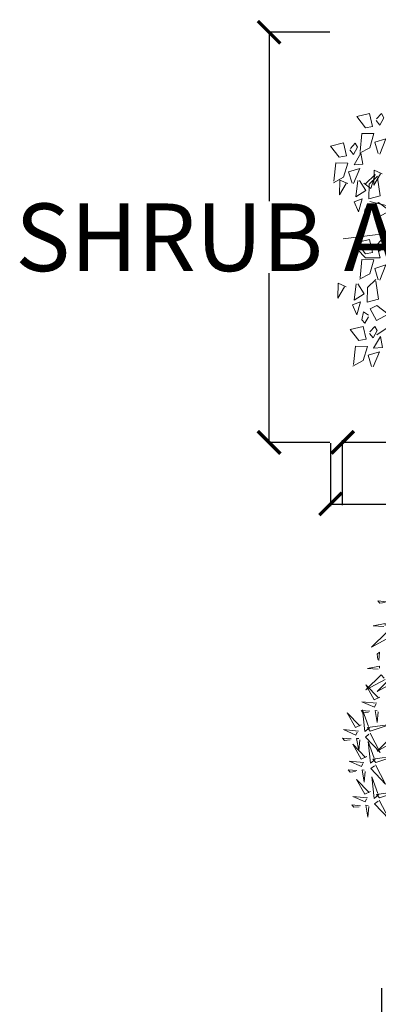
# Model space of a CAD drawing. Units: inches. Extents: x 1704 to 6393, y -157 to 1172.
# Tile 2 of 122: x 1866 to 1898, y -5 to 82. Entities that reach past the tile are written whole.
import ezdxf

# ---------------------------------------------------------------- set-up
doc = ezdxf.new("R2010")
doc.units = ezdxf.units.IN
doc.header["$MEASUREMENT"] = 0
for name, color, linetype, lineweight in [('A-ANNO-DIMS', 7, 'Continuous', 13), ('L-shrub', 74, 'Continuous', 18), ('L-tree', 102, 'Continuous', 18)]:
    doc.layers.add(name, color=color, linetype=linetype, lineweight=lineweight)
doc.styles.get("Standard").update_dxf_attribs({"font": 'arial.ttf'})
doc.dimstyles.get("Standard").update_dxf_attribs({"dimtxt": 6, "dimasz": 2, "dimexe": 0.18, "dimexo": 0.0625, "dimgap": 0.09, "dimtad": 0, "dimtih": 1, "dimtoh": 1, "dimdec": 1, "dimzin": 0, "dimdsep": 46, "dimlunit": 3, "dimtxsty": 'Standard', "dimblk": 'ARCHTICK', "dimcen": 0.09, "dimadec": 0, "dimazin": 0, "dimtfac": 1, "dimtdec": 1, "dimtofl": 0, "dimtmove": 0, "dimatfit": 3, "dimfxl": 1, "dimtolj": 1, "dimtzin": 0, "dimarcsym": 0})

# ---------------------------------------------------------------- blocks, each defined once
blk = doc.blocks.new('bamboo')
at = {"layer": 'L-shrub'}
for points in [[(-549.8, -1084.4), (-473.4, -1224.8), (-583.8, -1113.5), (-558.3, -1091.7)], [(-222.2, -1043.5), (-145.8, -1183.9), (-256.1, -1072.6), (-230.7, -1050.8)], [(214.7, -1043.5), (291.1, -1183.9), (180.8, -1072.6), (206.2, -1050.8)], [(376.8, -1193.4), (327.4, -1045.8), (350.9, -1214.7), (376.8, -1193.4)], [(636.2, -1166.1), (586.8, -1018.5), (610.3, -1187.4), (636.2, -1166.1)], [(-807.6, -1115.7), (-813.6, -1178.6), (-796.4, -1164.4), (-800.5, -1124.4)], [(-624.9, -1134.2), (-630.9, -1213), (-648, -1124.6), (-632.2, -1125.7)], [(-235.8, -1125.3), (-159.4, -1265.7), (-269.7, -1154.4), (-244.3, -1132.6)], [(144.7, -1234.3), (95.3, -1086.7), (118.8, -1255.6), (144.7, -1234.3)], [(392.5, -1194.9), (534.4, -1121.4), (420.9, -1229.4), (399.6, -1203.5)], [(651.9, -1167.6), (793.8, -1094.1), (680.3, -1202.1), (659, -1176.3)], [(-373.9, -1170.4), (-436.9, -1165.7), (-422.4, -1182.6), (-382.4, -1177.7)], [(-310.9, -1175.1), (-316.9, -1253.9), (-334, -1165.5), (-318.2, -1166.6)], [(-106.2, -1164.9), (-86.3, -1206.5), (-195.3, -1267.4), (-99.1, -1173.5)], [(-60.5, -1185.2), (-71, -1295.3), (-30.6, -1204), (-53.4, -1193.8)], [(3.9, -1175.6), (82.5, -1183.2), (-6.2, -1198.4), (-4.7, -1182.7)], [(160.4, -1235.8), (302.3, -1162.3), (188.8, -1270.3), (167.5, -1244.4)], [(352.4, -1199), (380.9, -1233.5), (220.7, -1249.7), (343.8, -1206.1)], [(611.8, -1171.7), (640.3, -1206.2), (480.1, -1222.4), (603.2, -1178.8)], [(120.3, -1239.9), (148.8, -1274.4), (-11.4, -1290.6), (111.7, -1247)], [(-2.1, -1238.5), (-8.1, -1301.4), (9.1, -1287.1), (5, -1247.1)], [(98.6, -1301.3), (118.4, -1342.9), (9.5, -1403.7), (105.7, -1309.9)], [(330.7, -1260.4), (350.5, -1301.9), (241.6, -1362.8), (337.8, -1269)], [(376.4, -1280.6), (365.9, -1390.7), (406.3, -1299.4), (383.5, -1289.3)], [(440.8, -1271), (519.4, -1278.6), (430.7, -1293.8), (432.2, -1278.1)], [(590.1, -1233.1), (609.9, -1274.7), (501, -1335.5), (597.2, -1241.7)], [(635.8, -1253.4), (625.3, -1363.4), (665.7, -1272.1), (642.9, -1262)], [(700.2, -1243.7), (778.8, -1251.3), (690.1, -1266.6), (691.6, -1250.8)], [(144.3, -1321.5), (133.8, -1431.6), (174.2, -1340.3), (151.4, -1330.2)], [(202.7, -1374.8), (196.7, -1437.7), (213.9, -1423.5), (209.8, -1383.4)], [(208.7, -1311.9), (287.3, -1319.5), (198.6, -1334.7), (200.1, -1319)], [(434.8, -1333.9), (428.8, -1396.8), (446, -1382.6), (441.9, -1342.5)], [(694.2, -1306.6), (688.2, -1369.5), (705.4, -1355.3), (701.3, -1315.3)]]:
    blk.add_lwpolyline(points, dxfattribs=at)
blk = doc.blocks.new('flower shrub 3')
at = {"layer": 'L-shrub'}
for p, q in [((10.1, -195.8), (26, -191.4)), ((14.6, -220.7), (10.1, -195.8)), ((26, -191.4), (25.9, -211.7)), ((25.9, -211.7), (14.5, -223))]:
    blk.add_line(p, q, dxfattribs=at)
for points in [[(-2.5, -5.1), (-51.6, -205.9)], [(7.3, -10), (132.3, -196.1)], [(-12.3, -147.2), (-0.1, -242.7)], [(-163.4, -197.2), (-157.2, -192), (-167.4, -186.6), (-173, -189.7), (-165.6, -196.5)], [(-117.8, -194.2), (-133.4, -199), (-138.2, -183.5), (-117.2, -192.1)], [(-89.9, -188.6), (-94.8, -199.8), (-74.4, -200.3), (-90, -190.9)], [(-50.4, -193.8), (-38.7, -178.3), (-30.1, -194.3), (-46.1, -202.9), (-50.4, -193.8)], [(10.5, -197.2), (16.8, -192), (6.6, -186.6), (1, -189.7), (8.3, -196.5)], [(56.1, -194.2), (40.6, -199), (35.8, -183.5), (56.8, -192.1)], [(91.9, -196.1), (103.6, -180.6), (112.3, -196.6), (96.2, -205.2), (91.9, -196.1)], [(150.8, -200.5), (149.6, -188.4), (134.7, -191.1), (150.8, -200.5)], [(-153.6, -211.9), (-169, -223.8), (-173.1, -206.1), (-155.4, -201.9), (-153.6, -211.9)], [(-120.5, -219.3), (-145.6, -216.6), (-145.5, -200.2), (-126, -205.9), (-118.3, -219.9)], [(-77, -213.9), (-69.5, -204.4), (-88.9, -198.6), (-76.3, -211.7)], [(-84.3, -195.1), (-59.4, -191.3), (-55.3, -207.2), (-75.6, -206.7), (-86.6, -195.1)], [(20.3, -211.9), (5, -223.8), (0.8, -206.1), (18.5, -201.9), (20.3, -211.9)], [(53.4, -219.3), (28.3, -216.6), (28.5, -200.2), (48, -205.9), (55.6, -219.9)], [(58, -197.4), (83, -193.6), (87.1, -209.5), (66.7, -208.9), (55.7, -197.3)], [(130.2, -206.2), (136.5, -201), (126.3, -195.6), (120.7, -198.7), (128.1, -205.6)], [(175.9, -203.3), (160.3, -208.1), (155.5, -192.5), (176.5, -201.1)], [(-102.2, -227.6), (-103.4, -215.5), (-118.3, -218.1), (-102.2, -227.6)], [(-80.5, -220.1), (-66.7, -211.4), (-58, -225.2), (-80.5, -222.3)], [(-55.5, -216.2), (-51.3, -227.6), (-37.6, -221.2), (-55.5, -216.2)], [(-37.1, -205.4), (-41.8, -212.1), (-30.6, -214.6), (-26, -210.3), (-34.9, -205.5)], [(61.8, -222.3), (75.6, -213.7), (84.3, -227.4), (61.8, -224.6)], [(105.2, -207.7), (100.5, -214.3), (111.7, -216.9), (116.3, -212.5), (107.4, -207.8)], [(140, -220.9), (124.7, -232.8), (120.5, -215.1), (138.3, -210.9), (140, -220.9)], [(173.2, -228.3), (148, -225.6), (148.2, -209.2), (167.7, -214.9), (175.3, -229)], [(-122.8, -233.3), (-116.5, -228.1), (-126.7, -222.7), (-132.3, -225.8), (-124.9, -232.6)], [(-77.1, -230.3), (-92.7, -235.1), (-97.5, -219.6), (-76.5, -228.2)], [(86.8, -218.5), (91, -229.9), (104.7, -223.5), (86.8, -218.5)], [(-113, -248), (-128.3, -259.9), (-132.5, -242.2), (-114.7, -238), (-113, -248)], [(-79.8, -255.4), (-105, -252.7), (-104.8, -236.3), (-85.3, -242), (-77.7, -256)], [(-76.4, -236), (-81.2, -247.1), (-60.9, -247.7), (-76.4, -238.2)], [(65.9, -238.2), (61.1, -249.4), (81.4, -249.9), (65.9, -240.5)]]:
    blk.add_lwpolyline(points, dxfattribs=at)
blk = doc.blocks.new('_ArchTick')
at = {"color": 0, "linetype": 'ByBlock', "const_width": 0.15}
blk.add_lwpolyline([(-0.5, -0.5), (0.5, 0.5)], dxfattribs=at)
blk = doc.blocks.new('*D71')
at = {"layer": 'A-ANNO-DIMS', "color": 0, "lineweight": -2, "transparency": 16777216}
for p, q in [((1894.896, 38.988), (1894.896, 44.734)), ((1894.896, 44.554), (1908.656, 44.554)), ((1931.183, 44.554), (1917.422, 44.554)), ((1931.183, 38.988), (1931.183, 44.734))]:
    blk.add_line(p, q, dxfattribs=at)
at = {"layer": 'Defpoints', "color": 0, "lineweight": -3, "transparency": 16777216}
for p in [(1931.183, 44.554), (1894.896, 38.926), (1931.183, 38.926)]:
    blk.add_point(p, dxfattribs=at)
at = {"layer": 'A-ANNO-DIMS', "color": 0, "lineweight": -2, "transparency": 16777216, "xscale": 2, "yscale": 2, "zscale": 2, "rotation": 180}
blk.add_blockref('_ArchTick', (1894.896, 44.554), dxfattribs=at)
at = {"layer": 'A-ANNO-DIMS', "color": 0, "lineweight": -2, "transparency": 16777216, "xscale": 2, "yscale": 2, "zscale": 2}
blk.add_blockref('_ArchTick', (1931.183, 44.554), dxfattribs=at)
at = {"layer": 'A-ANNO-DIMS', "color": 0, "transparency": 16777216, "insert": (1913.039, 44.554), "char_height": 6, "attachment_point": 5}
blk.add_mtext('\\A1;36', dxfattribs=at)
blk = doc.blocks.new('*D86')
at = {"layer": 'A-ANNO-DIMS', "color": 0, "lineweight": -2, "transparency": 16777216}
for p, q in [((1893.767, 80.936), (1888.19, 80.936)), ((1888.37, 80.936), (1888.37, 65.933)), ((1888.37, 44.542), (1888.37, 59.544)), ((1893.767, 44.542), (1888.19, 44.542))]:
    blk.add_line(p, q, dxfattribs=at)
at = {"layer": 'Defpoints', "color": 0, "lineweight": -3, "transparency": 16777216}
for p in [(1893.829, 80.936), (1888.37, 44.542), (1893.829, 44.542)]:
    blk.add_point(p, dxfattribs=at)
at = {"layer": 'A-ANNO-DIMS', "color": 0, "lineweight": -2, "transparency": 16777216, "xscale": 2, "yscale": 2, "zscale": 2}
for p, rotation in [((1888.37, 80.936), 90), ((1888.37, 44.542), 270)]:
    blk.add_blockref('_ArchTick', p, dxfattribs=dict(at, rotation=rotation))
at = {"layer": 'A-ANNO-DIMS', "color": 0, "transparency": 16777216, "insert": (1888.37, 62.739), "char_height": 6, "attachment_point": 5}
blk.add_mtext('\\A1;SHRUB A 36', dxfattribs=at)
blk = doc.blocks.new('*D87')
at = {"layer": 'A-ANNO-DIMS', "color": 0, "lineweight": -2, "transparency": 16777216}
for p, q in [((1893.829, 44.479), (1893.829, 38.903)), ((1928.523, 44.479), (1928.523, 38.903)), ((1893.829, 39.083), (1906.768, 39.083)), ((1928.523, 39.083), (1915.584, 39.083))]:
    blk.add_line(p, q, dxfattribs=at)
at = {"layer": 'Defpoints', "color": 0, "lineweight": -3, "transparency": 16777216}
for p in [(1893.829, 44.542), (1928.523, 44.542), (1928.523, 39.083)]:
    blk.add_point(p, dxfattribs=at)
at = {"layer": 'A-ANNO-DIMS', "color": 0, "lineweight": -2, "transparency": 16777216, "xscale": 2, "yscale": 2, "zscale": 2, "rotation": 180}
blk.add_blockref('_ArchTick', (1893.829, 39.083), dxfattribs=at)
at = {"layer": 'A-ANNO-DIMS', "color": 0, "lineweight": -2, "transparency": 16777216, "xscale": 2, "yscale": 2, "zscale": 2}
blk.add_blockref('_ArchTick', (1928.523, 39.083), dxfattribs=at)
at = {"layer": 'A-ANNO-DIMS', "color": 0, "transparency": 16777216, "insert": (1911.176, 39.083), "char_height": 6, "attachment_point": 5}
blk.add_mtext('\\A1;35', dxfattribs=at)
blk = doc.blocks.new('*D90')
at = {"layer": 'A-ANNO-DIMS', "color": 0, "lineweight": -2, "transparency": 16777216}
for p, q in [((1898.349, -3.85), (1898.349, -64.967)), ((2723.349, -3.85), (2723.349, -64.967)), ((1898.349, -64.787), (2304.104, -64.787)), ((2723.349, -64.787), (2317.593, -64.787))]:
    blk.add_line(p, q, dxfattribs=at)
at = {"layer": 'Defpoints', "color": 0, "lineweight": -3, "transparency": 16777216}
for p in [(1898.349, -3.787), (2723.349, -3.787), (2723.349, -64.787)]:
    blk.add_point(p, dxfattribs=at)
at = {"layer": 'A-ANNO-DIMS', "color": 0, "lineweight": -2, "transparency": 16777216, "xscale": 2, "yscale": 2, "zscale": 2, "rotation": 180}
blk.add_blockref('_ArchTick', (1898.349, -64.787), dxfattribs=at)
at = {"layer": 'A-ANNO-DIMS', "color": 0, "lineweight": -2, "transparency": 16777216, "xscale": 2, "yscale": 2, "zscale": 2}
blk.add_blockref('_ArchTick', (2723.349, -64.787), dxfattribs=at)
at = {"layer": 'A-ANNO-DIMS', "color": 0, "transparency": 16777216, "insert": (2310.849, -64.787), "char_height": 6, "attachment_point": 5}
blk.add_mtext('\\A1;825', dxfattribs=at)

msp = doc.modelspace()

# ---------------------------------------------------------------- block references
at = {"layer": 'L-shrub', "xscale": 0.0642956299502212, "yscale": 0.0642956299502212, "zscale": 0.0642956299502212, "rotation": 270}
msp.add_blockref('flower shrub 3', (1910.539, 62.588), dxfattribs=at)
at = {"layer": 'L-tree', "xscale": 0.0120554306156665, "yscale": 0.0120554306156665, "zscale": 0.0120554306156665, "rotation": 270}
msp.add_blockref('bamboo', (1912.228, 20.683), dxfattribs=at)

# ---------------------------------------------------------------- dimensions: what is measured, and where the dimension line sits
at = {"layer": 'A-ANNO-DIMS'}
dim = msp.add_linear_dim(base=(1888.37, 44.542), p1=(1893.829, 80.936), p2=(1893.829, 44.542), angle=270, text='SHRUB A <>', dimstyle='Standard', override={"dimdec": 0, "dimlfac": 1, "dimrnd": 0, "dimzin": 0, "dimdsep": 46, "dimlunit": 2}, dxfattribs=at)
dim.commit()
dim.dimension.update_dxf_attribs({"geometry": '*D86', "text_midpoint": (1888.37, 62.739)})
for base, p1, p2, picture, middle in [((1931.183, 44.554), (1894.896, 38.926), (1931.183, 38.926), '*D71', (1913.039, 44.554)), ((1928.523, 39.083), (1893.829, 44.542), (1928.523, 44.542), '*D87', (1911.176, 39.083)), ((2723.349, -64.787), (1898.349, -3.787), (2723.349, -3.787), '*D90', (2310.849, -64.787))]:
    dim = msp.add_linear_dim(base=base, p1=p1, p2=p2, dimstyle='Standard', override={"dimdec": 0, "dimlfac": 1, "dimrnd": 0, "dimzin": 0, "dimdsep": 46, "dimlunit": 2}, dxfattribs=at)
    dim.commit()
    dim.dimension.update_dxf_attribs({"geometry": picture, "text_midpoint": middle})

doc.saveas('drawing.dxf')
